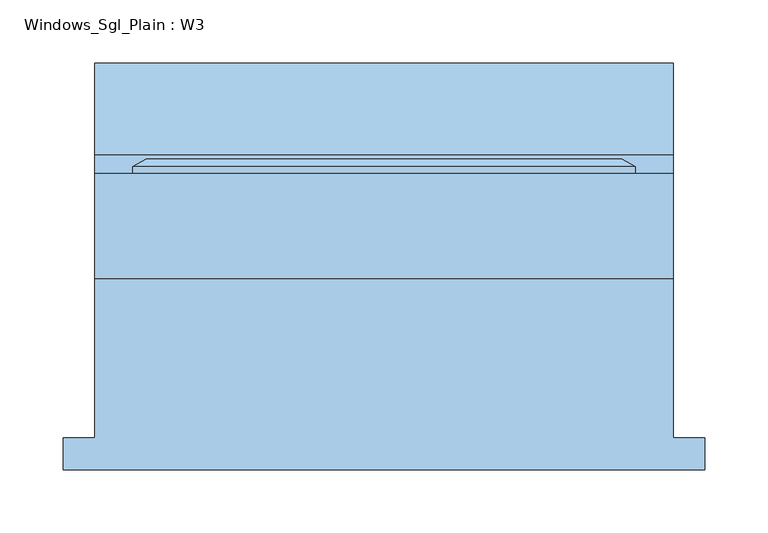
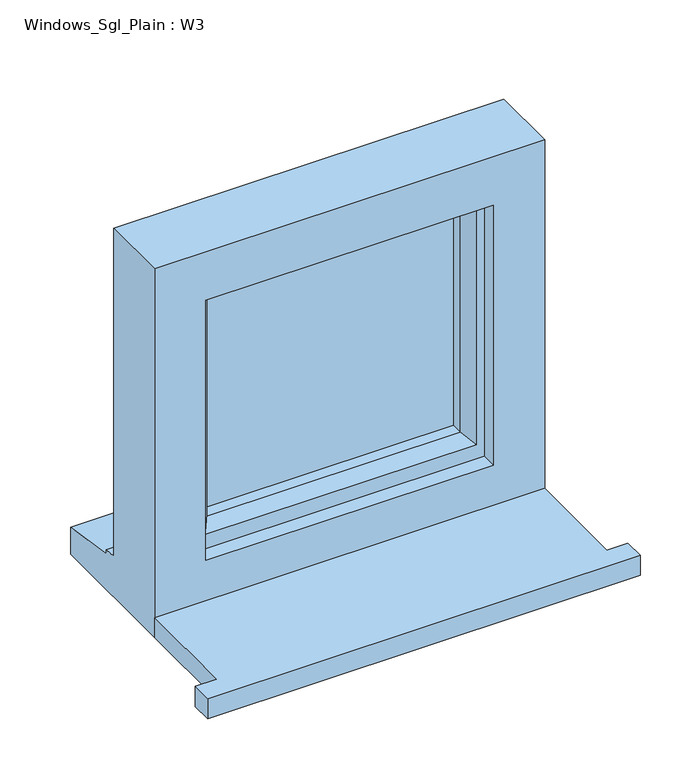
"""IFC4 building model written with IfcOpenShell, lengths in millimetres: window geometry, Windows_Sgl_Plain : W3."""

from ifc_helpers import new_model, si_unit, frame, origin, place, context, project, spatial, polyline, outline, extrude, faceted_brep, source, transform, mapped, element, save


def windows_sgl_plain_w3_b14593de(model_context):
    return source(origin(), model_context, "Body", "SolidModel", [
        extrude(outline(polyline([(-253.6, -146.0834322), (-253.6, -121.0834322), (-228.6, -121.0834322), (-228.6, 4.9965678), (228.6, 4.9965678), (228.6, -121.0834322), (253.6, -121.0834322), (253.6, -146.0834322), (-253.6, -146.0834322)])), frame((0.0, 0.0, 1652.8), z_axis=(0.0, 0.0, 1.0), x_axis=(1.0, 0.0, 0.0)), (0.0, 0.0, 1.0), 25.0),
        faceted_brep([(-228.6, 4.9965678, 1652.8), (228.6, 4.9965678, 1652.8), (228.6, 4.9965678, 2110.0), (-228.6, 4.9965678, 2110.0), (-168.6, 4.9965678, 2050.0), (168.6, 4.9965678, 2050.0), (168.6, 4.9965678, 1727.8), (-168.6, 4.9965678, 1727.8), (-228.6, 87.9965678, 2110.0), (-228.6, 87.9965678, 1703.8), (-228.6, 102.9965678, 1702.48767), (-228.6, 102.9965678, 1697.5449676), (-228.6, 175.4965678, 1686.6088847), (-228.6, 175.4965678, 1652.8), (228.6, 87.9965678, 2110.0), (228.6, 87.9965678, 1703.8), (-188.6, 87.9965678, 2070.0), (-188.6, 87.9965678, 1715.8), (188.6, 87.9965678, 1715.8), (188.6, 87.9965678, 2070.0), (-188.6, 22.9965678, 2070.0), (-188.6, 22.9965678, 1715.8), (188.6, 22.9965678, 2070.0), (188.6, 22.9965678, 1715.8), (-168.6, 22.9965678, 2050.0), (-168.6, 22.9965678, 1727.8), (168.6, 22.9965678, 1727.8), (168.6, 22.9965678, 2050.0), (228.6, 175.4965678, 1652.8), (228.6, 175.4965678, 1686.6088847), (228.6, 102.9965678, 1697.5449676), (228.6, 102.9965678, 1702.48767)], [[[0, 1, 2, 3], [4, 5, 6, 7]], [[0, 3, 8, 9, 10, 11, 12, 13]], [[9, 8, 14, 15], [16, 17, 18, 19]], [[17, 16, 20, 21]], [[20, 22, 23, 21], [24, 25, 26, 27]], [[24, 4, 7, 25]], [[3, 2, 14, 8]], [[16, 19, 22, 20]], [[5, 4, 24, 27]], [[15, 14, 2, 1, 28, 29, 30, 31]], [[19, 18, 23, 22]], [[5, 27, 26, 6]], [[28, 1, 0, 13]], [[29, 28, 13, 12]], [[30, 29, 12, 11]], [[31, 30, 11, 10]], [[15, 31, 10, 9]], [[21, 23, 18, 17]], [[7, 6, 26, 25]]]),
        extrude(outline(polyline([(158.6, 51.9965678), (-158.6, 51.9965678), (-158.6, 75.9965678), (158.6, 75.9965678), (158.6, 51.9965678)])), frame((0.0, 0.0, 1745.8), z_axis=(0.0, 0.0, 1.0), x_axis=(1.0, 0.0, 0.0)), (0.0, 0.0, 1.0), 294.2),
        faceted_brep([(-198.6, 87.9965678, 2080.0), (-198.6, 93.7700705, 2080.0), (-198.6, 93.7700705, 1705.8), (-198.6, 87.9965678, 1705.8), (-188.6, 22.9965678, 2070.0), (-188.6, 87.9965678, 2070.0), (-188.6, 87.9965678, 1715.8), (-188.6, 22.9965678, 1715.8), (-148.6, 37.4894677, 2030.0), (-158.7480377, 22.9965678, 2040.1480377), (-158.7480377, 22.9965678, 1745.6519623), (-148.6, 37.4894677, 1755.8), (-148.6, 51.9965678, 2030.0), (-148.6, 51.9965678, 1755.8), (-158.6, 75.9965678, 2040.0), (-158.6, 51.9965678, 2040.0), (-158.6, 51.9965678, 1745.8), (-158.6, 75.9965678, 1745.8), (-148.6, 93.7700705, 2030.0), (-148.6, 75.9965678, 2030.0), (-148.6, 75.9965678, 1755.8), (-148.6, 93.7700705, 1755.8), (-166.0457548, 99.5435732, 2047.4457548), (-166.0457548, 99.5435732, 1738.3542452), (-187.8153903, 99.5435732, 2069.2153903), (-187.8153903, 99.5435732, 1716.5846097), (198.6, 93.7700705, 1705.8), (198.6, 87.9965678, 1705.8), (188.6, 87.9965678, 1715.8), (188.6, 22.9965678, 1715.8), (158.7480377, 22.9965678, 1745.6519623), (148.6, 37.4894677, 1755.8), (148.6, 51.9965678, 1755.8), (158.6, 51.9965678, 1745.8), (158.6, 75.9965678, 1745.8), (148.6, 75.9965678, 1755.8), (148.6, 93.7700705, 1755.8), (166.0457548, 99.5435732, 1738.3542452), (187.8153903, 99.5435732, 1716.5846097), (198.6, 93.7700705, 2080.0), (198.6, 87.9965678, 2080.0), (188.6, 87.9965678, 2070.0), (188.6, 22.9965678, 2070.0), (158.7480377, 22.9965678, 2040.1480377), (148.6, 37.4894677, 2030.0), (148.6, 51.9965678, 2030.0), (158.6, 51.9965678, 2040.0), (158.6, 75.9965678, 2040.0), (148.6, 75.9965678, 2030.0), (148.6, 93.7700705, 2030.0), (166.0457548, 99.5435732, 2047.4457548), (187.8153903, 99.5435732, 2069.2153903)], [[[0, 1, 2, 3]], [[4, 5, 6, 7]], [[8, 9, 10, 11]], [[12, 8, 11, 13]], [[14, 15, 16, 17]], [[18, 19, 20, 21]], [[22, 18, 21, 23]], [[1, 24, 25, 2]], [[3, 2, 26, 27]], [[7, 6, 28, 29]], [[11, 10, 30, 31]], [[13, 11, 31, 32]], [[17, 16, 33, 34]], [[21, 20, 35, 36]], [[23, 21, 36, 37]], [[2, 25, 38, 26]], [[27, 26, 39, 40]], [[29, 28, 41, 42]], [[31, 30, 43, 44]], [[32, 31, 44, 45]], [[34, 33, 46, 47]], [[36, 35, 48, 49]], [[37, 36, 49, 50]], [[26, 38, 51, 39]], [[40, 39, 1, 0]], [[3, 27, 40, 0], [5, 41, 28, 6]], [[42, 41, 5, 4]], [[7, 29, 42, 4], [9, 43, 30, 10]], [[44, 43, 9, 8]], [[45, 44, 8, 12]], [[15, 46, 33, 16], [13, 32, 45, 12]], [[47, 46, 15, 14]], [[17, 34, 47, 14], [19, 48, 35, 20]], [[49, 48, 19, 18]], [[50, 49, 18, 22]], [[24, 51, 38, 25], [23, 37, 50, 22]], [[39, 51, 24, 1]]]),
    ])


if __name__ == "__main__":
    model = new_model("IFC4")
    model_context = context("Model", 3, world=origin())
    ifc_project = project(units=[si_unit("LENGTHUNIT", "METRE", prefix="MILLI")], contexts=[model_context])
    site = spatial("IfcSite", under=ifc_project)
    building = spatial("IfcBuilding", under=site)
    placement = place(None, origin())
    windows_sgl_plain_w3_shape = windows_sgl_plain_w3_b14593de(model_context)
    element("IfcWindow", 1, ObjectType="Windows_Sgl_Plain : W3", at=placement, inside=building, context=model_context, shape_type="MappedRepresentation", body=[
        mapped(windows_sgl_plain_w3_shape, transform((0.0, 0.0, 0.0), x_axis=(1.0, 0.0, 0.0), y_axis=(0.0, 1.0, 0.0), z_axis=(0.0, 0.0, 1.0))),
    ])
    save(model, "model.ifc")

# Revit data of these elements
# Type "Windows_Sgl_Plain : W3"
#   Type Mark = "58"
#   Operation = "SinglePanel"
#   Construction Type Id = "SGL"
#   Manufacturer = "Revit"
#   Keynote = "L10"
#   Analytic Construction = "Large single-glazed windows"
#   Wrap Layers (Ext) from Ext = 0.336286 ft
#   Wrap Layers (Int) from Ext = 0.582349 ft
#   Window Board Projection = 0.082021 ft
#   Window Board Extension = 0.082021 ft
#   Visual Light Transmittance = 0.9
#   Solar Heat Gain Coefficient = 0.86
#   Rough Width = 1.5 ft
#   Rough Height = 1.5 ft
#   Height = 1.5 ft
#   Width = 1.5 ft
#   Heat Transfer Coefficient (U) = 5.5617 W/(m²·K)
#   Glazing Thickness = 0.07874 ft
#   FrameOffset - External = 0.164042 ft
#   Frame Depth = 0.213255 ft
#   Default Head Height = 6.922572 ft
#   Cill Depth = 0.287073 ft
#   Cavity Closer Width = 0.164042 ft
#   Cavity Closer Offset from Ext = 0.336286 ft
#   Cavity Closer Depth = 0.278871 ft
#   Vis - Cavity Closers = yes
#   Define Thermal Properties by = 1
#   Material Trim = Window Frame
#   Material Glass = Glass
#   Material Frame = Window Frame
#   Wall Closure = (empty or 0)
# Element 1 (IfcWindow, "Windows_Sgl_Plain : W3")
#   Materials on its faces: "Window Frame", "Glass"
# Materials
#   "Window Frame": colour RGB 249 249 249, transparency 0, Keynote = "L10", Cost = 0
#   "Glass": class "Glass", colour RGB 0 128 192, transparency 0.9, Description = "Soda Lime Glass", Cost = 0
